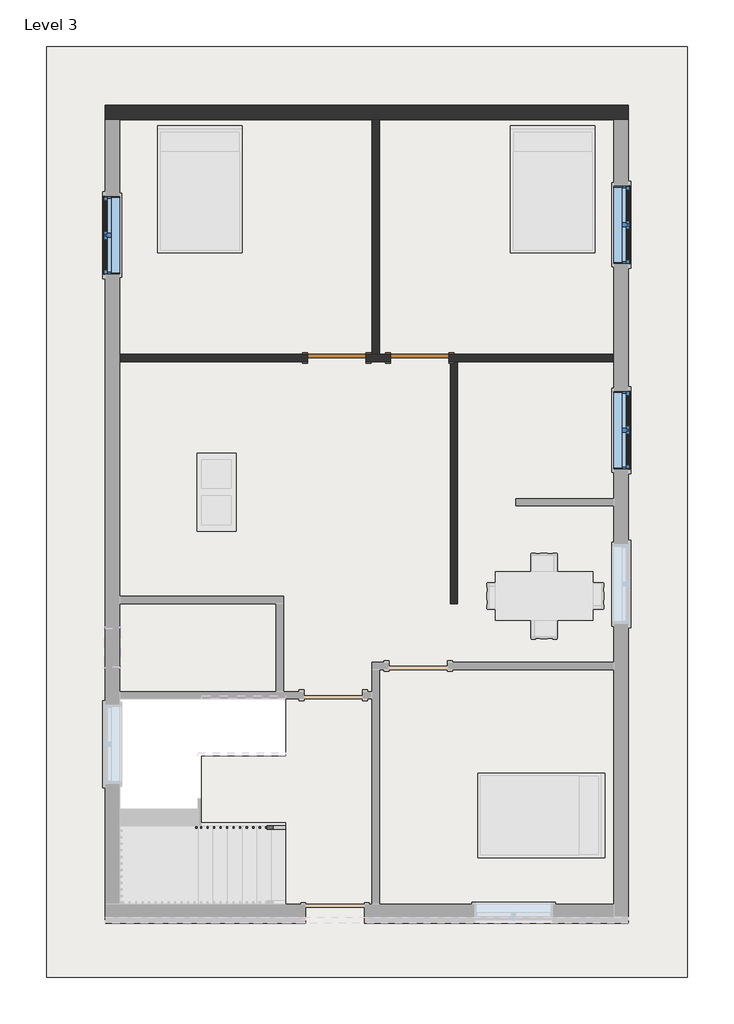
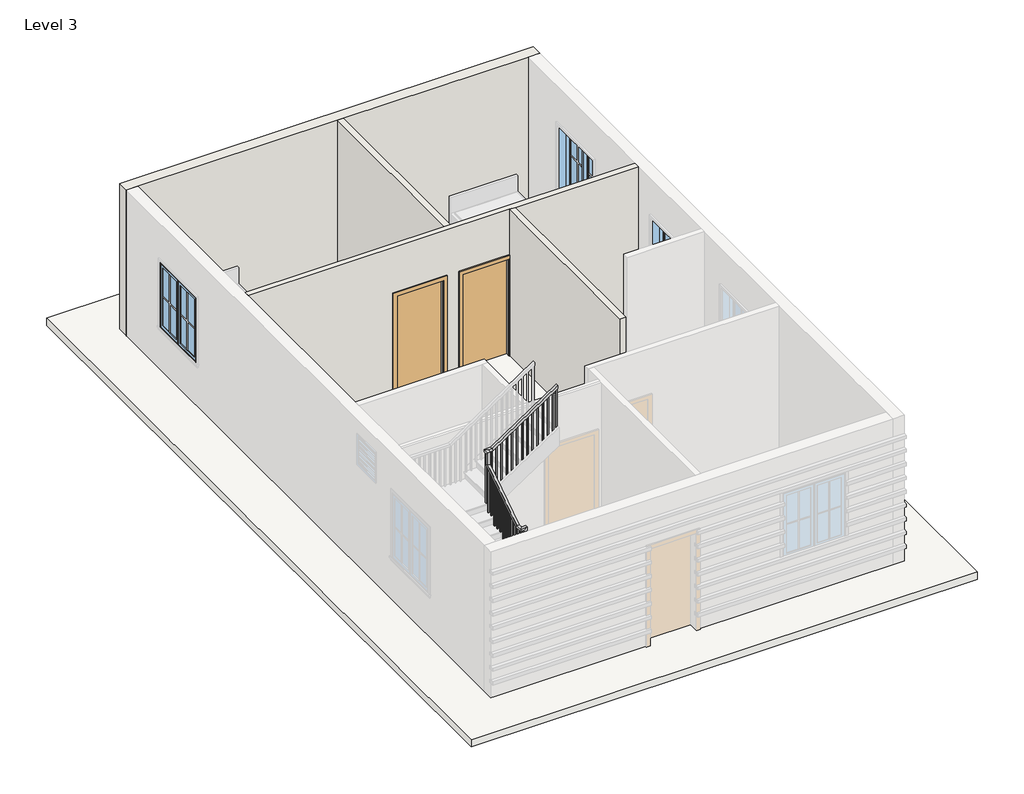
# One storey, part 2 of 3: 4 walls, 3 windows, 2 doors, 1 railing, 1 roof.
"""IFC4 building model written with IfcOpenShell, lengths in millimetres."""

from ifc_helpers import new_model, si_unit, frame, origin, place, context, project, spatial, polyline, outline, extrude, faceted_brep, transform, mapped, element, save
from components import single_flush_door_3_17d80c48, single_flush_door_3_5e62189b, window_casement_double_window_4_576b2d2c

model = new_model("IFC4")

# Units and contexts
model_context = context("Model", 3, world=origin())
ifc_project = project(units=[si_unit("LENGTHUNIT", "METRE", prefix="MILLI")], contexts=[model_context])

# Site, building, storey
site = spatial("IfcSite", under=ifc_project)
building = spatial("IfcBuilding", under=site)
storey = spatial("IfcBuildingStorey", under=building, Name="Level 3", Elevation=6248.4)

# Doors
placement = place(None, origin())
single_flush_door_3_shape = single_flush_door_3_17d80c48(model_context)
element("IfcDoor", 1, ObjectType="Single-Flush : DOOR 3'", at=placement, inside=storey, context=model_context, shape_type="MappedRepresentation", body=[
    mapped(single_flush_door_3_shape, transform((-1721.4617403, 2133.1073441, 6248.4), x_axis=(1.0, 0.0, 0.0), y_axis=(0.0, 1.0, 0.0), z_axis=(0.0, 0.0, 1.0))),
])
single_flush_door_3_2_shape = single_flush_door_3_5e62189b(model_context)
element("IfcDoor", 2, ObjectType="Single-Flush : DOOR 3'", at=placement, inside=storey, context=model_context, shape_type="MappedRepresentation", body=[
    mapped(single_flush_door_3_2_shape, transform((-426.0617403, 2133.1073441, 6248.4), x_axis=(-1.0, 0.0, 0.0), y_axis=(0.0, -1.0, 0.0), z_axis=(0.0, 0.0, 1.0))),
])

# Railing
element("IfcRailing", 3, ObjectType="Handrail - Rectangular", at=placement, inside=storey, context=model_context, shape_type="SolidModel", body=[
    faceted_brep([(-2515.2117403, -5213.8426559, 7315.2), (-2515.2117403, -5213.8426559, 7254.1459984), (-2515.2117403, -5163.0426559, 7254.1459984), (-2515.2117403, -5163.0426559, 7315.2), (-3810.6117403, -5213.8426559, 8178.8), (-3861.4117403, -5213.8426559, 8151.6126651), (-3861.4117403, -5163.0426559, 8151.6126651), (-3810.6117403, -5163.0426559, 8178.8), (-3810.6117403, -5213.8426559, 8432.8), (-3861.4117403, -5213.8426559, 8382.0), (-3861.4117403, -5163.0426559, 8382.0), (-3810.6117403, -5163.0426559, 8432.8), (-3937.6117403, -5213.8426559, 8432.8), (-3937.6117403, -5213.8426559, 8382.0), (-3886.8117403, -5163.0426559, 8382.0), (-3886.8117403, -5163.0426559, 8432.8), (-3937.6117403, -5086.8426559, 8432.8), (-3937.6117403, -5071.4616535, 8382.0), (-3886.8117403, -5071.4616535, 8382.0), (-3886.8117403, -5086.8426559, 8432.8), (-3937.6117403, -4096.2426559, 9093.2), (-3937.6117403, -4045.4426559, 9066.0126651), (-3886.8117403, -4045.4426559, 9066.0126651), (-3886.8117403, -4096.2426559, 9093.2), (-3937.6117403, -4096.2426559, 9347.2), (-3937.6117403, -4045.4426559, 9296.4), (-3886.8117403, -4045.4426559, 9296.4), (-3886.8117403, -4096.2426559, 9347.2), (-3937.6117403, -3969.2426559, 9347.2), (-3937.6117403, -3969.2426559, 9296.4), (-3886.8117403, -4020.0426559, 9296.4), (-3886.8117403, -4020.0426559, 9347.2), (-3810.6117403, -3969.2426559, 9347.2), (-3795.2307379, -3969.2426559, 9296.4), (-3795.2307379, -4020.0426559, 9296.4), (-3810.6117403, -4020.0426559, 9347.2), (-2515.2117403, -3969.2426559, 10210.8), (-2515.2117403, -4020.0426559, 10210.8), (-2515.2117403, -4020.0426559, 10149.7459984), (-2515.2117403, -3969.2426559, 10149.7459984)], [[[0, 1, 2, 3]], [[1, 0, 4, 5]], [[2, 1, 5, 6]], [[3, 2, 6, 7]], [[0, 3, 7, 4]], [[5, 4, 8, 9]], [[6, 5, 9, 10]], [[7, 6, 10, 11]], [[4, 7, 11, 8]], [[9, 8, 12, 13]], [[10, 9, 13, 14]], [[11, 10, 14, 15]], [[8, 11, 15, 12]], [[13, 12, 16, 17]], [[14, 13, 17, 18]], [[15, 14, 18, 19]], [[12, 15, 19, 16]], [[17, 16, 20, 21]], [[18, 17, 21, 22]], [[19, 18, 22, 23]], [[16, 19, 23, 20]], [[21, 20, 24, 25]], [[22, 21, 25, 26]], [[23, 22, 26, 27]], [[20, 23, 27, 24]], [[25, 24, 28, 29]], [[26, 25, 29, 30]], [[27, 26, 30, 31]], [[24, 27, 31, 28]], [[29, 28, 32, 33]], [[30, 29, 33, 34]], [[31, 30, 34, 35]], [[28, 31, 35, 32]], [[36, 37, 38, 39]], [[33, 32, 36, 39]], [[34, 33, 39, 38]], [[35, 34, 38, 37]], [[32, 35, 37, 36]]]),
    extrude(outline(polyline([(10105.2959984, -2581.8867403), (10092.5959984, -2600.9367403), (9144.0, -2600.9367403), (9144.0, -2581.8867403), (10105.2959984, -2581.8867403)])), frame((0.0, -4004.1676559, 0.0), z_axis=(0.0, 1.0, 0.0), x_axis=(0.0, 0.0, 1.0)), (0.0, 0.0, 1.0), 19.05),
    extrude(outline(polyline([(10037.5626651, -2683.4867403), (10024.8626651, -2702.5367403), (9144.0, -2702.5367403), (9144.0, -2683.4867403), (10037.5626651, -2683.4867403)])), frame((0.0, -4004.1676559, 0.0), z_axis=(0.0, 1.0, 0.0), x_axis=(0.0, 0.0, 1.0)), (0.0, 0.0, 1.0), 19.05),
    extrude(outline(polyline([(9969.8293317, -2785.0867403), (9957.1293317, -2804.1367403), (8991.6, -2804.1367403), (8991.6, -2785.0867403), (9969.8293317, -2785.0867403)])), frame((0.0, -4004.1676559, 0.0), z_axis=(0.0, 1.0, 0.0), x_axis=(0.0, 0.0, 1.0)), (0.0, 0.0, 1.0), 19.05),
    extrude(outline(polyline([(9902.0959984, -2886.6867403), (9889.3959984, -2905.7367403), (8991.6, -2905.7367403), (8991.6, -2886.6867403), (9902.0959984, -2886.6867403)])), frame((0.0, -4004.1676559, 0.0), z_axis=(0.0, 1.0, 0.0), x_axis=(0.0, 0.0, 1.0)), (0.0, 0.0, 1.0), 19.05),
    extrude(outline(polyline([(9834.3626651, -2988.2867403), (9821.6626651, -3007.3367403), (8839.2, -3007.3367403), (8839.2, -2988.2867403), (9834.3626651, -2988.2867403)])), frame((0.0, -4004.1676559, 0.0), z_axis=(0.0, 1.0, 0.0), x_axis=(0.0, 0.0, 1.0)), (0.0, 0.0, 1.0), 19.05),
    extrude(outline(polyline([(9766.6293317, -3089.8867403), (9753.9293317, -3108.9367403), (8839.2, -3108.9367403), (8839.2, -3089.8867403), (9766.6293317, -3089.8867403)])), frame((0.0, -4004.1676559, 0.0), z_axis=(0.0, 1.0, 0.0), x_axis=(0.0, 0.0, 1.0)), (0.0, 0.0, 1.0), 19.05),
    extrude(outline(polyline([(9698.8959984, -3191.4867403), (9686.1959984, -3210.5367403), (8839.2, -3210.5367403), (8839.2, -3191.4867403), (9698.8959984, -3191.4867403)])), frame((0.0, -4004.1676559, 0.0), z_axis=(0.0, 1.0, 0.0), x_axis=(0.0, 0.0, 1.0)), (0.0, 0.0, 1.0), 19.05),
    extrude(outline(polyline([(9631.1626651, -3293.0867403), (9618.4626651, -3312.1367403), (8686.8, -3312.1367403), (8686.8, -3293.0867403), (9631.1626651, -3293.0867403)])), frame((0.0, -4004.1676559, 0.0), z_axis=(0.0, 1.0, 0.0), x_axis=(0.0, 0.0, 1.0)), (0.0, 0.0, 1.0), 19.05),
    extrude(outline(polyline([(9563.4293317, -3394.6867403), (9550.7293317, -3413.7367403), (8686.8, -3413.7367403), (8686.8, -3394.6867403), (9563.4293317, -3394.6867403)])), frame((0.0, -4004.1676559, 0.0), z_axis=(0.0, 1.0, 0.0), x_axis=(0.0, 0.0, 1.0)), (0.0, 0.0, 1.0), 19.05),
    extrude(outline(polyline([(9495.6959984, -3496.2867403), (9482.9959984, -3515.3367403), (8534.4, -3515.3367403), (8534.4, -3496.2867403), (9495.6959984, -3496.2867403)])), frame((0.0, -4004.1676559, 0.0), z_axis=(0.0, 1.0, 0.0), x_axis=(0.0, 0.0, 1.0)), (0.0, 0.0, 1.0), 19.05),
    extrude(outline(polyline([(9427.9626651, -3597.8867403), (9415.2626651, -3616.9367403), (8534.4, -3616.9367403), (8534.4, -3597.8867403), (9427.9626651, -3597.8867403)])), frame((0.0, -4004.1676559, 0.0), z_axis=(0.0, 1.0, 0.0), x_axis=(0.0, 0.0, 1.0)), (0.0, 0.0, 1.0), 19.05),
    extrude(outline(polyline([(9360.2293317, -3699.4867403), (9347.5293317, -3718.5367403), (8382.0, -3718.5367403), (8382.0, -3699.4867403), (9360.2293317, -3699.4867403)])), frame((0.0, -4004.1676559, 0.0), z_axis=(0.0, 1.0, 0.0), x_axis=(0.0, 0.0, 1.0)), (0.0, 0.0, 1.0), 19.05),
    extrude(outline(polyline([(9292.4959984, -3801.0867403), (9279.7959984, -3820.1367403), (8382.0, -3820.1367403), (8382.0, -3801.0867403), (9292.4959984, -3801.0867403)])), frame((0.0, -4004.1676559, 0.0), z_axis=(0.0, 1.0, 0.0), x_axis=(0.0, 0.0, 1.0)), (0.0, 0.0, 1.0), 19.05),
    extrude(outline(polyline([(-3902.6867403, -4080.3676559), (-3921.7367403, -4080.3676559), (-3921.7367403, -4061.3176559), (-3902.6867403, -4061.3176559), (-3902.6867403, -4080.3676559)])), frame((0.0, 0.0, 8077.2), z_axis=(0.0, 0.0, 1.0), x_axis=(1.0, 0.0, 0.0)), (0.0, 0.0, 1.0), 1219.2),
    extrude(outline(polyline([(-4181.9676559, 8974.9959984), (-4162.9176559, 8987.6959984), (-4162.9176559, 8077.2), (-4181.9676559, 8077.2), (-4181.9676559, 8974.9959984)])), frame((-3921.7367403, 0.0, 0.0), z_axis=(1.0, 0.0, 0.0), x_axis=(0.0, 1.0, 0.0)), (0.0, 0.0, 1.0), 19.05),
    extrude(outline(polyline([(-4283.5676559, 8907.2626651), (-4264.5176559, 8919.9626651), (-4264.5176559, 7924.8), (-4283.5676559, 7924.8), (-4283.5676559, 8907.2626651)])), frame((-3921.7367403, 0.0, 0.0), z_axis=(1.0, 0.0, 0.0), x_axis=(0.0, 1.0, 0.0)), (0.0, 0.0, 1.0), 19.05),
    extrude(outline(polyline([(-4385.1676559, 8839.5293317), (-4366.1176559, 8852.2293317), (-4366.1176559, 7924.8), (-4385.1676559, 7924.8), (-4385.1676559, 8839.5293317)])), frame((-3921.7367403, 0.0, 0.0), z_axis=(1.0, 0.0, 0.0), x_axis=(0.0, 1.0, 0.0)), (0.0, 0.0, 1.0), 19.05),
    extrude(outline(polyline([(-4486.7676559, 8771.7959984), (-4467.7176559, 8784.4959984), (-4467.7176559, 7924.8), (-4486.7676559, 7924.8), (-4486.7676559, 8771.7959984)])), frame((-3921.7367403, 0.0, 0.0), z_axis=(1.0, 0.0, 0.0), x_axis=(0.0, 1.0, 0.0)), (0.0, 0.0, 1.0), 19.05),
    extrude(outline(polyline([(-4588.3676559, 8704.0626651), (-4569.3176559, 8716.7626651), (-4569.3176559, 7772.4), (-4588.3676559, 7772.4), (-4588.3676559, 8704.0626651)])), frame((-3921.7367403, 0.0, 0.0), z_axis=(1.0, 0.0, 0.0), x_axis=(0.0, 1.0, 0.0)), (0.0, 0.0, 1.0), 19.05),
    extrude(outline(polyline([(-4689.9676559, 8636.3293317), (-4670.9176559, 8649.0293317), (-4670.9176559, 7772.4), (-4689.9676559, 7772.4), (-4689.9676559, 8636.3293317)])), frame((-3921.7367403, 0.0, 0.0), z_axis=(1.0, 0.0, 0.0), x_axis=(0.0, 1.0, 0.0)), (0.0, 0.0, 1.0), 19.05),
    extrude(outline(polyline([(-4791.5676559, 8568.5959984), (-4772.5176559, 8581.2959984), (-4772.5176559, 7620.0), (-4791.5676559, 7620.0), (-4791.5676559, 8568.5959984)])), frame((-3921.7367403, 0.0, 0.0), z_axis=(1.0, 0.0, 0.0), x_axis=(0.0, 1.0, 0.0)), (0.0, 0.0, 1.0), 19.05),
    extrude(outline(polyline([(-4893.1676559, 8500.8626651), (-4874.1176559, 8513.5626651), (-4874.1176559, 7620.0), (-4893.1676559, 7620.0), (-4893.1676559, 8500.8626651)])), frame((-3921.7367403, 0.0, 0.0), z_axis=(1.0, 0.0, 0.0), x_axis=(0.0, 1.0, 0.0)), (0.0, 0.0, 1.0), 19.05),
    extrude(outline(polyline([(-4994.7676559, 8433.1293317), (-4975.7176559, 8445.8293317), (-4975.7176559, 7467.6), (-4994.7676559, 7467.6), (-4994.7676559, 8433.1293317)])), frame((-3921.7367403, 0.0, 0.0), z_axis=(1.0, 0.0, 0.0), x_axis=(0.0, 1.0, 0.0)), (0.0, 0.0, 1.0), 19.05),
    extrude(outline(polyline([(-5096.3676559, 8365.3959984), (-5077.3176559, 8378.0959984), (-5077.3176559, 7467.6), (-5096.3676559, 7467.6), (-5096.3676559, 8365.3959984)])), frame((-3921.7367403, 0.0, 0.0), z_axis=(1.0, 0.0, 0.0), x_axis=(0.0, 1.0, 0.0)), (0.0, 0.0, 1.0), 19.05),
    extrude(outline(polyline([(-3826.4867403, -5178.9176559), (-3826.4867403, -5197.9676559), (-3845.5367403, -5197.9676559), (-3845.5367403, -5178.9176559), (-3826.4867403, -5178.9176559)])), frame((0.0, 0.0, 7162.8), z_axis=(0.0, 0.0, 1.0), x_axis=(1.0, 0.0, 0.0)), (0.0, 0.0, 1.0), 1219.2),
    extrude(outline(polyline([(8060.5959984, -3724.8867403), (8073.2959984, -3743.9367403), (7162.8, -3743.9367403), (7162.8, -3724.8867403), (8060.5959984, -3724.8867403)])), frame((0.0, -5197.9676559, 0.0), z_axis=(0.0, 1.0, 0.0), x_axis=(0.0, 0.0, 1.0)), (0.0, 0.0, 1.0), 19.05),
    extrude(outline(polyline([(7992.8626651, -3623.2867403), (8005.5626651, -3642.3367403), (7010.4, -3642.3367403), (7010.4, -3623.2867403), (7992.8626651, -3623.2867403)])), frame((0.0, -5197.9676559, 0.0), z_axis=(0.0, 1.0, 0.0), x_axis=(0.0, 0.0, 1.0)), (0.0, 0.0, 1.0), 19.05),
    extrude(outline(polyline([(7925.1293317, -3521.6867403), (7937.8293317, -3540.7367403), (7010.4, -3540.7367403), (7010.4, -3521.6867403), (7925.1293317, -3521.6867403)])), frame((0.0, -5197.9676559, 0.0), z_axis=(0.0, 1.0, 0.0), x_axis=(0.0, 0.0, 1.0)), (0.0, 0.0, 1.0), 19.05),
    extrude(outline(polyline([(7857.3959984, -3420.0867403), (7870.0959984, -3439.1367403), (7010.4, -3439.1367403), (7010.4, -3420.0867403), (7857.3959984, -3420.0867403)])), frame((0.0, -5197.9676559, 0.0), z_axis=(0.0, 1.0, 0.0), x_axis=(0.0, 0.0, 1.0)), (0.0, 0.0, 1.0), 19.05),
    extrude(outline(polyline([(7789.6626651, -3318.4867403), (7802.3626651, -3337.5367403), (6858.0, -3337.5367403), (6858.0, -3318.4867403), (7789.6626651, -3318.4867403)])), frame((0.0, -5197.9676559, 0.0), z_axis=(0.0, 1.0, 0.0), x_axis=(0.0, 0.0, 1.0)), (0.0, 0.0, 1.0), 19.05),
    extrude(outline(polyline([(7721.9293317, -3216.8867403), (7734.6293317, -3235.9367403), (6858.0, -3235.9367403), (6858.0, -3216.8867403), (7721.9293317, -3216.8867403)])), frame((0.0, -5197.9676559, 0.0), z_axis=(0.0, 1.0, 0.0), x_axis=(0.0, 0.0, 1.0)), (0.0, 0.0, 1.0), 19.05),
    extrude(outline(polyline([(7654.1959984, -3115.2867403), (7666.8959984, -3134.3367403), (6705.6, -3134.3367403), (6705.6, -3115.2867403), (7654.1959984, -3115.2867403)])), frame((0.0, -5197.9676559, 0.0), z_axis=(0.0, 1.0, 0.0), x_axis=(0.0, 0.0, 1.0)), (0.0, 0.0, 1.0), 19.05),
    extrude(outline(polyline([(7586.4626651, -3013.6867403), (7599.1626651, -3032.7367403), (6705.6, -3032.7367403), (6705.6, -3013.6867403), (7586.4626651, -3013.6867403)])), frame((0.0, -5197.9676559, 0.0), z_axis=(0.0, 1.0, 0.0), x_axis=(0.0, 0.0, 1.0)), (0.0, 0.0, 1.0), 19.05),
    extrude(outline(polyline([(7518.7293317, -2912.0867403), (7531.4293317, -2931.1367403), (6553.2, -2931.1367403), (6553.2, -2912.0867403), (7518.7293317, -2912.0867403)])), frame((0.0, -5197.9676559, 0.0), z_axis=(0.0, 1.0, 0.0), x_axis=(0.0, 0.0, 1.0)), (0.0, 0.0, 1.0), 19.05),
    extrude(outline(polyline([(7450.9959984, -2810.4867403), (7463.6959984, -2829.5367403), (6553.2, -2829.5367403), (6553.2, -2810.4867403), (7450.9959984, -2810.4867403)])), frame((0.0, -5197.9676559, 0.0), z_axis=(0.0, 1.0, 0.0), x_axis=(0.0, 0.0, 1.0)), (0.0, 0.0, 1.0), 19.05),
    extrude(outline(polyline([(7383.2626651, -2708.8867403), (7395.9626651, -2727.9367403), (6400.8, -2727.9367403), (6400.8, -2708.8867403), (7383.2626651, -2708.8867403)])), frame((0.0, -5197.9676559, 0.0), z_axis=(0.0, 1.0, 0.0), x_axis=(0.0, 0.0, 1.0)), (0.0, 0.0, 1.0), 19.05),
    extrude(outline(polyline([(7315.5293317, -2607.2867403), (7328.2293317, -2626.3367403), (6400.8, -2626.3367403), (6400.8, -2607.2867403), (7315.5293317, -2607.2867403)])), frame((0.0, -5197.9676559, 0.0), z_axis=(0.0, 1.0, 0.0), x_axis=(0.0, 0.0, 1.0)), (0.0, 0.0, 1.0), 19.05),
    extrude(outline(polyline([(-3902.6867403, -4004.1676559), (-3921.7367403, -4004.1676559), (-3921.7367403, -3985.1176559), (-3902.6867403, -3985.1176559), (-3902.6867403, -4004.1676559)])), frame((0.0, 0.0, 8229.6), z_axis=(0.0, 0.0, 1.0), x_axis=(1.0, 0.0, 0.0)), (0.0, 0.0, 1.0), 1066.8),
    extrude(outline(polyline([(-3902.6867403, -5178.9176559), (-3902.6867403, -5197.9676559), (-3921.7367403, -5197.9676559), (-3921.7367403, -5178.9176559), (-3902.6867403, -5178.9176559)])), frame((0.0, 0.0, 7315.2), z_axis=(0.0, 0.0, 1.0), x_axis=(1.0, 0.0, 0.0)), (0.0, 0.0, 1.0), 1066.8),
    extrude(outline(polyline([(10149.7459984, -2515.2117403), (10137.0459984, -2534.2617403), (9144.0, -2534.2617403), (9144.0, -2515.2117403), (10149.7459984, -2515.2117403)])), frame((0.0, -4004.1676559, 0.0), z_axis=(0.0, 1.0, 0.0), x_axis=(0.0, 0.0, 1.0)), (0.0, 0.0, 1.0), 19.05),
    extrude(outline(polyline([(7254.1459984, -2515.2117403), (7266.8459984, -2534.2617403), (6400.8, -2534.2617403), (6400.8, -2515.2117403), (7254.1459984, -2515.2117403)])), frame((0.0, -5197.9676559, 0.0), z_axis=(0.0, 1.0, 0.0), x_axis=(0.0, 0.0, 1.0)), (0.0, 0.0, 1.0), 19.05),
])

# Roof
element("IfcRoof", 4, ObjectType="ROOF 6\"", at=placement, inside=storey, context=model_context, shape_type="SweptSolid", body=[
    extrude(outline(polyline([(-6249.0117403, -7525.2426559), (-6249.0117403, 6990.8573441), (3745.8882597, 6990.8573441), (3745.8882597, -7525.2426559), (-6249.0117403, -7525.2426559)]), holes=[polyline([(-5156.8117403, -3131.0426559), (-5156.8117403, -6433.0426559), (-2515.2117403, -6433.0426559), (-2515.2117403, -5112.2426559), (-3836.0117403, -5112.2426559), (-3836.0117403, -4070.8426559), (-2515.2117403, -4070.8426559), (-2515.2117403, -3131.0426559), (-5156.8117403, -3131.0426559)])]), frame((0.0, 0.0, 6096.0), z_axis=(0.0, 0.0, 1.0), x_axis=(1.0, 0.0, 0.0)), (0.0, 0.0, 1.0), 152.4),
])

# Walls
element("IfcWall", 5, ObjectType="ALL 4.5\"", at=placement, inside=storey, context=model_context, shape_type="Brep", body=[
    faceted_brep([(-1264.2617403, 2075.9573441, 6248.4), (-883.2617403, 2075.9573441, 6248.4), (-883.2617403, 2075.9573441, 8280.4), (31.1382597, 2075.9573441, 8280.4), (31.1382597, 2075.9573441, 6248.4), (50.1882597, 2075.9573441, 6248.4), (164.4882597, 2075.9573441, 6248.4), (2602.8882597, 2075.9573441, 6248.4), (2602.8882597, 2075.9573441, 9296.4), (164.4882597, 2075.9573441, 9296.4), (50.1882597, 2075.9573441, 9296.4), (-5106.0117403, 2075.9573441, 9296.4), (-5106.0117403, 2075.9573441, 6248.4), (-2178.6617403, 2075.9573441, 6248.4), (-2178.6617403, 2075.9573441, 8280.4), (-1264.2617403, 2075.9573441, 8280.4), (-883.2617403, 2190.2573441, 8280.4), (-883.2617403, 2190.2573441, 6248.4), (-1054.7117403, 2190.2573441, 6248.4), (-1169.0117403, 2190.2573441, 6248.4), (-1264.2617403, 2190.2573441, 6248.4), (-1264.2617403, 2190.2573441, 8280.4), (-2178.6617403, 2190.2573441, 8280.4), (-2178.6617403, 2190.2573441, 6248.4), (-5106.0117403, 2190.2573441, 6248.4), (-5106.0117403, 2190.2573441, 9296.4), (-1169.0117403, 2190.2573441, 9296.4), (-1054.7117403, 2190.2573441, 9296.4), (2602.8882597, 2190.2573441, 9296.4), (2602.8882597, 2190.2573441, 6248.4), (31.1382597, 2190.2573441, 6248.4), (31.1382597, 2190.2573441, 8280.4)], [[[0, 1, 2, 3, 4, 5, 6, 7, 8, 9, 10, 11, 12, 13, 14, 15]], [[16, 17, 18, 19, 20, 21, 22, 23, 24, 25, 26, 27, 28, 29, 30, 31]], [[13, 12, 24, 23]], [[30, 29, 7, 6, 5, 4]], [[20, 19, 18, 17, 1, 0]], [[8, 7, 29, 28]], [[12, 11, 25, 24]], [[21, 20, 0, 15]], [[22, 21, 15, 14]], [[23, 22, 14, 13]], [[2, 1, 17, 16]], [[3, 2, 16, 31]], [[4, 3, 31, 30]], [[11, 10, 9, 8, 28, 27, 26, 25]]]),
])
element("IfcWall", 6, ObjectType="ALL 4.5\"", at=placement, inside=storey, context=model_context, shape_type="SweptSolid", body=[
    extrude(outline(polyline([(50.1882597, -1695.9426559), (50.1882597, 2075.9573441), (164.4882597, 2075.9573441), (164.4882597, -1695.9426559), (50.1882597, -1695.9426559)])), frame((0.0, 0.0, 6248.4), z_axis=(0.0, 0.0, 1.0), x_axis=(1.0, 0.0, 0.0)), (0.0, 0.0, 1.0), 3048.0),
])
element("IfcWall", 7, ObjectType="ALL 4.5\"", at=placement, inside=storey, context=model_context, shape_type="SweptSolid", body=[
    extrude(outline(polyline([(-1169.0117403, 2190.2573441), (-1169.0117403, 5847.8573441), (-1054.7117403, 5847.8573441), (-1054.7117403, 2190.2573441), (-1169.0117403, 2190.2573441)])), frame((0.0, 0.0, 6248.4), z_axis=(0.0, 0.0, 1.0), x_axis=(1.0, 0.0, 0.0)), (0.0, 0.0, 1.0), 3048.0),
])
element("IfcWall", 8, ObjectType="WALL 9\"", at=placement, inside=storey, context=model_context, shape_type="Brep", body=[
    faceted_brep([(-5334.6117403, 5847.8573441, 6248.4), (-5106.0117403, 5847.8573441, 6248.4), (-1169.0117403, 5847.8573441, 6248.4), (-1054.7117403, 5847.8573441, 6248.4), (2602.8882597, 5847.8573441, 6248.4), (2831.4882597, 5847.8573441, 6248.4), (2831.4882597, 5847.8573441, 9296.4), (2602.8882597, 5847.8573441, 9296.4), (-1054.7117403, 5847.8573441, 9296.4), (-1169.0117403, 5847.8573441, 9296.4), (-5106.0117403, 5847.8573441, 9296.4), (-5334.6117403, 5847.8573441, 9296.4), (-5334.6117403, 6076.4573441, 6248.4), (-5334.6117403, 6076.4573441, 9296.4), (2831.4882597, 6076.4573441, 9296.4), (2831.4882597, 6076.4573441, 6248.4)], [[[0, 1, 2, 3, 4, 5, 6, 7, 8, 9, 10, 11]], [[12, 13, 14, 15]], [[5, 4, 3, 2, 1, 0, 12, 15]], [[6, 5, 15, 14]], [[0, 11, 13, 12]], [[11, 10, 9, 8, 7, 6, 14, 13]]]),
])

# Windows
window_casement_double_window_4_shape = window_casement_double_window_4_576b2d2c(model_context)
element("IfcWindow", 9, ObjectType="Window-Casement-Double : WINDOW 4'", at=placement, inside=storey, context=model_context, shape_type="MappedRepresentation", body=[
    mapped(window_casement_double_window_4_shape, transform((-5220.3117403, 4047.6323441, 6248.4), x_axis=(0.0, 1.0, 0.0), y_axis=(-1.0, 0.0, 0.0), z_axis=(0.0, 0.0, 1.0))),
])
element("IfcWindow", 10, ObjectType="Window-Casement-Double : WINDOW 4'", at=placement, inside=storey, context=model_context, shape_type="MappedRepresentation", body=[
    mapped(window_casement_double_window_4_shape, transform((2717.1882597, 4209.5573441, 6248.4), x_axis=(0.0, -1.0, 0.0), y_axis=(1.0, 0.0, 0.0), z_axis=(0.0, 0.0, 1.0))),
])
element("IfcWindow", 11, ObjectType="Window-Casement-Double : WINDOW 4'", at=placement, inside=storey, context=model_context, shape_type="MappedRepresentation", body=[
    mapped(window_casement_double_window_4_shape, transform((2717.1882597, 1009.1573441, 6248.4), x_axis=(0.0, -1.0, 0.0), y_axis=(1.0, 0.0, 0.0), z_axis=(0.0, 0.0, 1.0))),
])

save(model, "model.ifc")

# Revit data of these elements
# Type "Single-Flush : DOOR 3'"
#   Type Mark = "8"
#   Construction Type Id = "MDOOR"
#   Assembly Code = "C1020"
#   Analytic Construction = "Metal"
#   Thickness = 0' - 2"
#   Heat Transfer Coefficient (U) = 0.651978 BTU/(h·ft²·°F)
#   Height = 6' - 8"
#   Trim Projection Ext = 0' - 1"
#   Trim Projection Int = 0' - 1"
#   Trim Width = 0' - 3"
#   Width = 3' - 0"
#   Define Thermal Properties by = 1
#   Door Material = Door - Panel
#   Frame Material = Door - Frame
#   Visual Light Transmittance = 0
#   Solar Heat Gain Coefficient = 0
#   Function = (empty or 0)
#   Wall Closure = (empty or 0)
# Type "Handrail - Rectangular"
#   Assembly Code = "C2010400"
#   built-in parameter 1008612 = 0.0416667 (stored number, unit not read)
#   built-in parameter 1008611 = 0.0416667 (stored number, unit not read)
#   built-in parameter 1008609 = 0.333333 (stored number, unit not read)
#   built-in parameter 1008604 = 0.166667 (stored number, unit not read)
#   built-in parameter 1008603 = 0.166667 (stored number, unit not read)
#   Railing Height = 3' - 0"
#   built-in parameter 1008630 = 2
#   built-in parameter 1008610 = 2
#   built-in parameter 1008618 = Baluster - Square : 3/4"
# Type "ROOF 6\""
#   Assembly Code = "B1020"
#   Layers, outside or top first: 0' - 6" no material (function 1)
# Type "ALL 4.5\""
#   Assembly Code = "B2010"
#   Layers, outside or top first: 0' - 4 1/2" no material (function 1)
# Type "WALL 9\""
#   Assembly Code = "B2010"
#   Layers, outside or top first: 0' - 9" "Carpet (1)" (function 1)
# Type "Window-Casement-Double : WINDOW 4'"
#   Type Mark = "18"
#   Fire Rating = "0.5h"
#   Assembly Code = "B2020100"
#   Analytic Construction = "Double glazing - domestic"
#   Frame Extension [instance default] = 0' - 0 1/4"
#   Window Inset [instance default] = 0' - 0"
#   Wall Thickness [instance default] = 0' - 6"
#   Interior Wall Closure [instance default] = 0' - 2 1/4"
#   Half Width = 2' - 0"
#   Visual Light Transmittance = 0.81
#   Thermal Resistance (R) = 1.8146 (h·ft²·°F)/BTU
#   Solar Heat Gain Coefficient = 0.76
#   Rough Width = 4' - 0 1/2"
#   Rough Height = 4' - 5 1/2"
#   Height = 4' - 5"
#   Heat Transfer Coefficient (U) = 0.5511 BTU/(h·ft²·°F)
#   Exterior Wall Closure [instance default] = 0' - 1 1/4"
#   Extension Jamb [instance default] = 0' - 2 1/4"
#   Default Sill Height = 3' - 0"
#   Width = 4' - 0"
#   Muntin Visibility = yes
#   Interior Trim Visibility [instance default] = yes
#   Exterior Trim Visibility [instance default] = yes
#   Extension Jamb Visibility [instance default] = yes
#   Interior Trim Material = Wood - Stained
#   Muntin Pattern = Muntin Pattern_2x2 : Muntin Pattern_2x2
#   Interior Trim = Trim-Window-Interior-Flat : Picture Frame
#   Interior Frame Material = Wood - Stained
#   Glass Panel Material = Glass
#   Exterior Trim Material = Clad - White
#   Exterior Trim = Trim-Window-Exterior-Flat : with Sill
#   Exterior Frame Material = Clad - White
#   Wall Closure = (empty or 0)
# Elements 1, 2 (IfcDoor, "Single-Flush : DOOR 3'")
#   Phase Created = New Construction
#   Materials on its faces: "Door - Frame", "Door - Panel"
# Element 3 (IfcRailing, "Handrail - Rectangular")
#   Phase Created = New Construction
#   Materials on its faces: "Clad - White"
# Element 4 (IfcRoof, "ROOF 6\"")
#   built-in parameter 1001705 = 20.5 (stored number, unit not read)
#   built-in parameter 1001701 = -0.5 (stored number, unit not read)
#   built-in parameter 1001710 = 33615
#   Phase Created = New Construction
#   Materials on its faces: "Clad - White", "Default Roof", "Softwood, Lumber"
# Elements 5, 6, 7 (IfcWall, "ALL 4.5\"")
#   Top Offset = 0' - 0"
#   Base Offset = 0' - 0"
#   Unconnected Height = 10' - 0"
#   wall height = 10' - 0"
#   Phase Created = New Construction
#   Base Constraint = Level 3
#   Materials on its faces: "Default Wall"
# Element 8 (IfcWall, "WALL 9\"")
#   Top Offset = 0' - 0"
#   Base Offset = 0' - 0"
#   Unconnected Height = 10' - 0"
#   wall height = 10' - 0"
#   Phase Created = New Construction
#   Base Constraint = Level 3
#   Materials on its faces: "Carpet (1)", "Wood - Stained"
# Element 9 (IfcWindow, "Window-Casement-Double : WINDOW 4'")
#   Mark = "16"
#   Window Inset = 0' - 0"
#   Interior Wall Closure = 0' - 2 1/4"
#   Frame Extension = 0' - 0 1/4"
#   Exterior Wall Closure = 0' - 1 1/4"
#   Interior Trim Visibility = yes
#   Exterior Trim Visibility = yes
#   Phase Created = New Construction
#   Materials on its faces: "Wood - Stained", "Glass", "Clad - White"
# Element 10 (IfcWindow, "Window-Casement-Double : WINDOW 4'")
#   Mark = "17"
#   Window Inset = 0' - 0"
#   Interior Wall Closure = 0' - 2 1/4"
#   Frame Extension = 0' - 0 1/4"
#   Exterior Wall Closure = 0' - 1 1/4"
#   Interior Trim Visibility = yes
#   Exterior Trim Visibility = yes
#   Phase Created = New Construction
#   Materials on its faces: "Wood - Stained", "Glass", "Clad - White"
# Element 11 (IfcWindow, "Window-Casement-Double : WINDOW 4'")
#   Mark = "18"
#   Window Inset = 0' - 0"
#   Interior Wall Closure = 0' - 2 1/4"
#   Frame Extension = 0' - 0 1/4"
#   Exterior Wall Closure = 0' - 1 1/4"
#   Interior Trim Visibility = yes
#   Exterior Trim Visibility = yes
#   Phase Created = New Construction
#   Materials on its faces: "Wood - Stained", "Glass", "Clad - White"
# Materials
#   "Door - Panel": class "Wood", colour RGB 210 159 95, transparency 0, Cost = 0
#   "Door - Frame": colour RGB 118 70 51, transparency 0, Cost = 0
#   "Carpet (1)": class "Carpet", colour RGB 124 80 67, transparency 0, Description = "Interior finish", Cost = 0
#   "Wood - Stained": class "Wood", colour RGB 224 178 126, transparency 0, Cost = 0
#   "Glass": class "Glass", colour RGB 0 128 192, transparency 0.75, Description = "Soda Lime Glass", Cost = 0
#   "Clad - White": class "Wood", colour RGB 242 242 238, transparency 0, Cost = 0
#   "Default Roof": colour RGB 88 101 114, transparency 0, Cost = 0
#   "Softwood, Lumber": class "Wood", colour RGB 223 192 134, transparency 0, Description = "Pinus Echinata", Cost = 0
#   "Default Wall": colour RGB 128 128 128, transparency 0, Cost = 0
